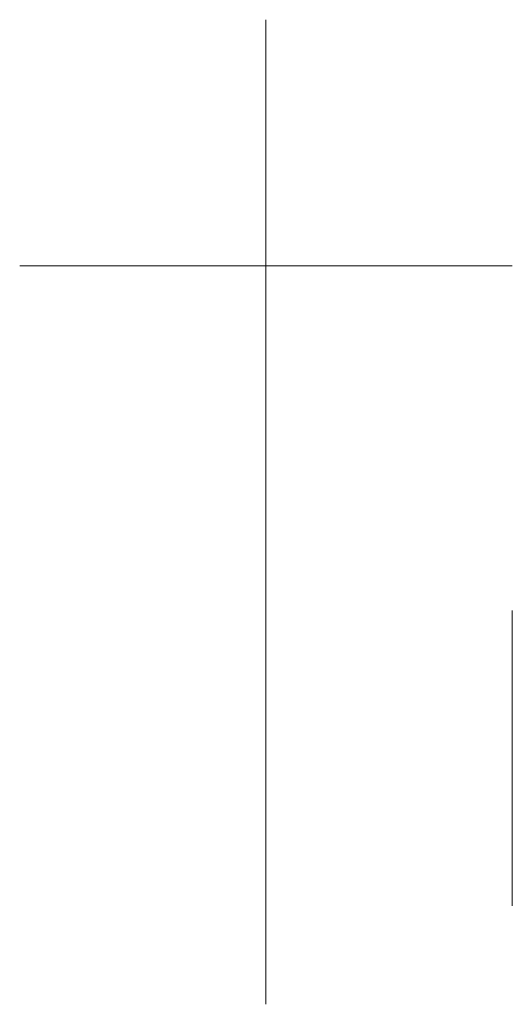
# Model space of a CAD drawing. Units: inches. Extents: x -10 to 10, y -112.4 to -72.4.
import ezdxf

# ---------------------------------------------------------------- set-up
doc = ezdxf.new("R2010")
doc.units = ezdxf.units.IN
doc.header["$MEASUREMENT"] = 0
doc.layers.add('M-CONS', color=8, linetype='Continuous', lineweight=13)

msp = doc.modelspace()

# ---------------------------------------------------------------- linework, layer by layer
at = {"layer": 'M-CONS'}
for p, q in [((0, -72.421, 1819.981), (0, -82.421, 1819.981)), ((0, -72.421, 1839.981), (0, -82.421, 1839.981)), ((0, -92.421, 1839.981), (0, -82.421, 1839.981))]:
    msp.add_line(p, q, dxfattribs=at)
at = {"layer": 'M-CONS', "extrusion": (0, -1, 0)}
msp.add_line((0, -72.421, 1819.981), (0, -92.421, 1819.981), dxfattribs=at)
at = {"layer": 'M-CONS', "extrusion": (1, 0, 0)}
msp.add_lwpolyline([(-72.421, 1839.981), (-102.421, 1839.981, 1), (-102.421, 1819.981), (-72.421, 1819.981)], format="xyb", close=True, dxfattribs=at)
at = {"layer": 'M-CONS', "extrusion": (0, -1, 0)}
msp.add_circle((0, 1859.981, 82.421), 10, dxfattribs=at)
at = {"layer": 'M-CONS', "extrusion": (1, -2.27e-14, 0)}
msp.add_circle((-102.421, 1829.981, 10), 6, dxfattribs=at)

doc.saveas('drawing.dxf')
